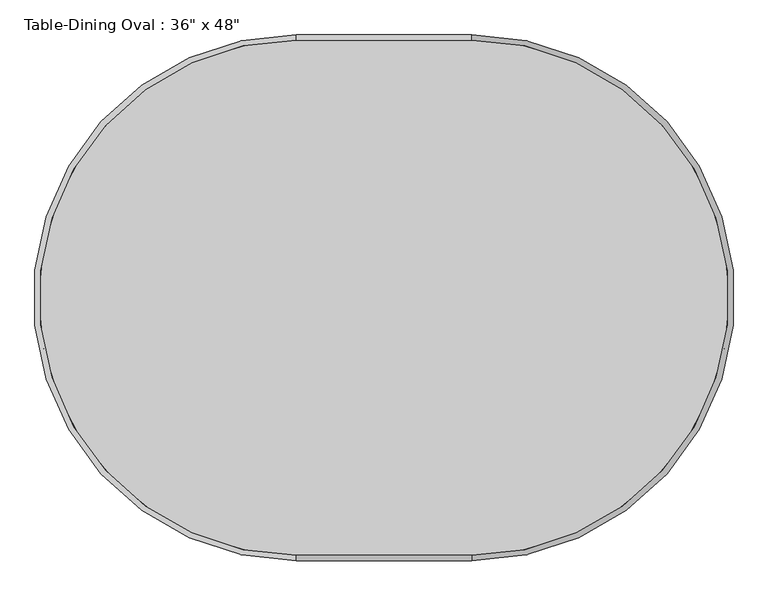
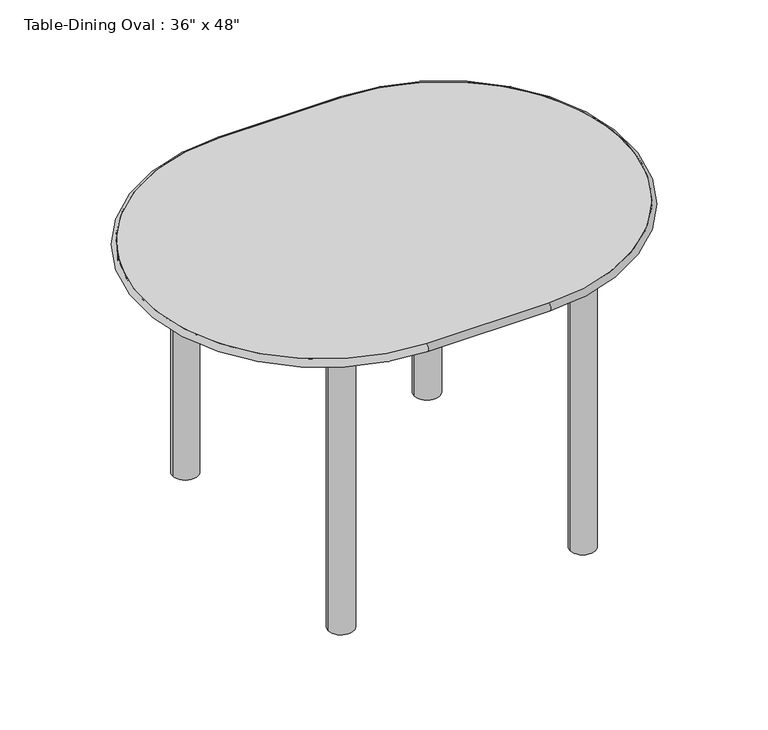
"""IFC4 building model written with IfcOpenShell, lengths in millimetres: furniture geometry."""

from ifc_helpers import new_model, si_unit, point, frame, frame_2d, origin, origin_with_axes, place, context, project, spatial, polyline, circle_curve, ellipse_curve, trimmed, segment, composite_curve, outline, extrude, source, transform, mapped, element, save
from ifc_brep_helpers import plane_surface, cylinder_surface, revolved_surface, advanced_brep


def furniture_be1c6672(model_context):
    return source(origin(), model_context, "Body", "SolidModel", [
        advanced_brep(
        [(-554.2196721, -805.7733607, 762.0), (-554.2196721, -805.7733607, 742.95), (-249.4196721, -805.7733607, 742.95), (-249.4196721, -805.7733607, 762.0), (-249.4196721, 89.5766393, 762.0), (-249.4196721, 89.5766393, 742.95), (-554.2196721, 89.5766393, 742.95), (-554.2196721, 89.5766393, 762.0)],
        [
            (0, 1, circle_curve(frame((-554.2196721, -805.7733607, 752.475), z_axis=(1.0, 0.0, 0.0), x_axis=(0.0, 1.0, 0.0)), 9.525)),
            (1, 2),
            (2, 3, circle_curve(frame((-249.4196721, -805.7733607, 752.475), z_axis=(-1.0, 0.0, 0.0), x_axis=(0.0, 1.0, 0.0)), 9.525)),
            (3, 0),
            (1, 0),
            (3, 2),
            (4, 3, circle_curve(frame((-249.4196721, -358.0983607, 762.0), z_axis=(0.0, 0.0, -1.0), x_axis=(0.0, -1.0, 0.0)), 447.675)),
            (2, 5, circle_curve(frame((-249.4196721, -358.0983607, 742.95), z_axis=(0.0, 0.0, 1.0), x_axis=(0.0, -1.0, 0.0)), 447.675)),
            (5, 4, circle_curve(frame((-249.4196721, 89.5766393, 752.475), z_axis=(1.0, 0.0, 0.0), x_axis=(0.0, -1.0, 0.0)), 9.525)),
            (4, 5),
            (5, 6),
            (6, 7, circle_curve(frame((-554.2196721, 89.5766393, 752.475), z_axis=(1.0, 0.0, 0.0), x_axis=(0.0, -1.0, 0.0)), 9.525)),
            (7, 4),
            (7, 6),
            (0, 7, circle_curve(frame((-554.2196721, -358.0983607, 762.0), z_axis=(0.0, 0.0, -1.0), x_axis=(0.0, 1.0, 0.0)), 447.675)),
            (6, 1, circle_curve(frame((-554.2196721, -358.0983607, 742.95), z_axis=(0.0, 0.0, 1.0), x_axis=(0.0, 1.0, 0.0)), 447.675)),
        ],
        [
            cylinder_surface(frame((-554.2196721, -805.7733607, 752.475), z_axis=(-1.0, 0.0, 0.0), x_axis=(0.0, 1.0, 0.0)), 9.525),
            plane_surface(frame((-554.2196721, -805.7733607, 762.0), z_axis=(0.0, 1.0, 0.0), x_axis=(1.0, 0.0, 0.0))),
            revolved_surface(trimmed(ellipse_curve(frame((-249.4196721, -805.7733607, 752.475), z_axis=(-1.0, 0.0, 0.0), x_axis=(0.0, 1.0, 0.0)), 9.525, 9.525), [point((-249.4196721, -805.7733607, 742.95))], [point((-249.4196721, -805.7733607, 762.0))], True, "CARTESIAN"), (-249.4196721, -358.0983607, 0.0), (0.0, 0.0, 1.0)),
            revolved_surface(polyline([(-249.4196721, -805.7733607, 762.0), (-249.4196721, -805.7733607, 742.95)]), (-249.4196721, -358.0983607, 0.0), (0.0, 0.0, 1.0)),
            cylinder_surface(frame((-249.4196721, 89.5766393, 752.475), z_axis=(1.0, 0.0, 0.0), x_axis=(0.0, -1.0, 0.0)), 9.525),
            plane_surface(frame((-249.4196721, 89.5766393, 762.0), z_axis=(0.0, -1.0, 0.0), x_axis=(-1.0, 0.0, 0.0))),
            revolved_surface(trimmed(ellipse_curve(frame((-554.2196721, 89.5766393, 752.475), z_axis=(1.0, 0.0, 0.0), x_axis=(0.0, -1.0, 0.0)), 9.525, 9.525), [point((-554.2196721, 89.5766393, 742.95))], [point((-554.2196721, 89.5766393, 762.0))], True, "CARTESIAN"), (-554.2196721, -358.0983607, 0.0), (0.0, 0.0, 1.0)),
            revolved_surface(polyline([(-554.2196721, 89.57663930000001, 762.0), (-554.2196721, 89.57663930000001, 742.95)]), (-554.2196721, -358.0983607, 0.0), (0.0, 0.0, 1.0)),
        ],
        [
            (0, [[1, 2, 3, 4]]),
            (1, [[5, -4, 6, -2]]),
            (2, [[7, -3, 8, 9]]),
            (3, [[-8, -6, -7, 10]]),
            (4, [[-9, 11, 12, 13]]),
            (5, [[-10, -13, 14, -11]]),
            (6, [[15, -12, 16, -1]]),
            (7, [[-16, -14, -15, -5]]),
        ],
    ),
        extrude(outline(composite_curve([segment(trimmed(circle_curve(frame_2d((-703.4446721, -21.5483607)), 31.75), [point((-735.1946721, -21.5483607))], [point((-671.6946721, -21.5483607))], False, "CARTESIAN"), True, "CONTINUOUS"), segment(trimmed(circle_curve(frame_2d((-703.4446721, -21.5483607)), 31.75), [point((-671.6946721, -21.5483607))], [point((-735.1946721, -21.5483607))], False, "CARTESIAN"), True, "CONTINUOUS")], self_intersect=False)), origin_with_axes(), (0.0, 0.0, 1.0), 742.95),
        extrude(outline(composite_curve([segment(trimmed(circle_curve(frame_2d((-703.4446721, -694.6483607)), 31.75), [point((-735.1946721, -694.6483607))], [point((-671.6946721, -694.6483607))], False, "CARTESIAN"), True, "CONTINUOUS"), segment(trimmed(circle_curve(frame_2d((-703.4446721, -694.6483607)), 31.75), [point((-671.6946721, -694.6483607))], [point((-735.1946721, -694.6483607))], False, "CARTESIAN"), True, "CONTINUOUS")], self_intersect=False)), origin_with_axes(), (0.0, 0.0, 1.0), 742.95),
        extrude(outline(composite_curve([segment(trimmed(circle_curve(frame_2d((-100.1946721, -21.5483607)), 31.75), [point((-131.9446721, -21.5483607))], [point((-68.4446721, -21.5483607))], False, "CARTESIAN"), True, "CONTINUOUS"), segment(trimmed(circle_curve(frame_2d((-100.1946721, -21.5483607)), 31.75), [point((-68.4446721, -21.5483607))], [point((-131.9446721, -21.5483607))], False, "CARTESIAN"), True, "CONTINUOUS")], self_intersect=False)), origin_with_axes(), (0.0, 0.0, 1.0), 742.95),
        extrude(outline(composite_curve([segment(trimmed(circle_curve(frame_2d((-100.1946721, -694.6483607)), 31.75), [point((-131.9446721, -694.6483607))], [point((-68.4446721, -694.6483607))], False, "CARTESIAN"), True, "CONTINUOUS"), segment(trimmed(circle_curve(frame_2d((-100.1946721, -694.6483607)), 31.75), [point((-68.4446721, -694.6483607))], [point((-131.9446721, -694.6483607))], False, "CARTESIAN"), True, "CONTINUOUS")], self_intersect=False)), origin_with_axes(), (0.0, 0.0, 1.0), 742.95),
        extrude(outline(polyline([(-81.1446721, -2.4983607), (-81.1446721, -713.6983607), (-722.4946721, -713.6983607), (-722.4946721, -2.4983607), (-81.1446721, -2.4983607)]), holes=[polyline([(-100.1946721, -21.5483607), (-703.4446721, -21.5483607), (-703.4446721, -694.6483607), (-100.1946721, -694.6483607), (-100.1946721, -21.5483607)])]), frame((0.0, 0.0, 692.15), z_axis=(0.0, 0.0, 1.0), x_axis=(1.0, 0.0, 0.0)), (0.0, 0.0, 1.0), 50.8),
        extrude(outline(composite_curve([segment(polyline([(-554.2196721, 89.5766393), (-249.4196721, 89.5766393)]), True, "CONTINUOUS"), segment(trimmed(circle_curve(frame_2d((-249.4196721, -358.0983607)), 447.675), [point((-249.4196721, 89.5766393))], [point((198.2553279, -358.0983607))], False, "CARTESIAN"), True, "CONTINUOUS"), segment(trimmed(circle_curve(frame_2d((-249.4196721, -358.0983607)), 447.675), [point((198.2553279, -358.0983607))], [point((-249.4196721, -805.7733607))], False, "CARTESIAN"), True, "CONTINUOUS"), segment(polyline([(-249.4196721, -805.7733607), (-554.2196721, -805.7733607)]), True, "CONTINUOUS"), segment(trimmed(circle_curve(frame_2d((-554.2196721, -358.0983607)), 447.675), [point((-554.2196721, -805.7733607))], [point((-1001.8946721, -358.0983607))], False, "CARTESIAN"), True, "CONTINUOUS"), segment(trimmed(circle_curve(frame_2d((-554.2196721, -358.0983607)), 447.675), [point((-1001.8946721, -358.0983607))], [point((-554.2196721, 89.5766393))], False, "CARTESIAN"), True, "CONTINUOUS")], self_intersect=False)), frame((0.0, 0.0, 742.95), z_axis=(0.0, 0.0, 1.0), x_axis=(1.0, 0.0, 0.0)), (0.0, 0.0, 1.0), 19.05),
    ])


if __name__ == "__main__":
    model = new_model("IFC4")
    model_context = context("Model", 3, world=origin())
    ifc_project = project(units=[si_unit("LENGTHUNIT", "METRE", prefix="MILLI")], contexts=[model_context])
    site = spatial("IfcSite", under=ifc_project)
    building = spatial("IfcBuilding", under=site)
    placement = place(None, origin())
    furniture_shape = furniture_be1c6672(model_context)
    element("IfcFurniture", 1, ObjectType="Table-Dining Oval : 36\" x 48\"", at=placement, inside=building, context=model_context, shape_type="MappedRepresentation", body=[
        mapped(furniture_shape, transform((0.0, 0.0, 0.0), x_axis=(1.0, 0.0, 0.0), y_axis=(0.0, 1.0, 0.0), z_axis=(0.0, 0.0, 1.0))),
    ])
    save(model, "model.ifc")

# Revit data of these elements
# Type "Table-Dining Oval : 36\" x 48\""
#   Assembly Code = "E2020200"
#   Length = 4' - 0"
#   Width = 3' - 0"
#   Base Material = Steel, Chrome Plated
#   Top Material = Glass - Clear, Grey
#   Default Elevation = 0
#   Description = (empty or 0)
# Element 1 (IfcFurniture, "Table-Dining Oval : 36\" x 48\"")
#   Materials on its faces: "Steel, Chrome Plated", "Glass - Clear, Grey"
# Materials
#   "Steel, Chrome Plated": class "Metal", colour RGB 17 17 17, transparency 0, Description = "Chromiuim plated steel", Cost = 0
#   "Glass - Clear, Grey": class "Glass", colour RGB 252 255 255, transparency 0.64
